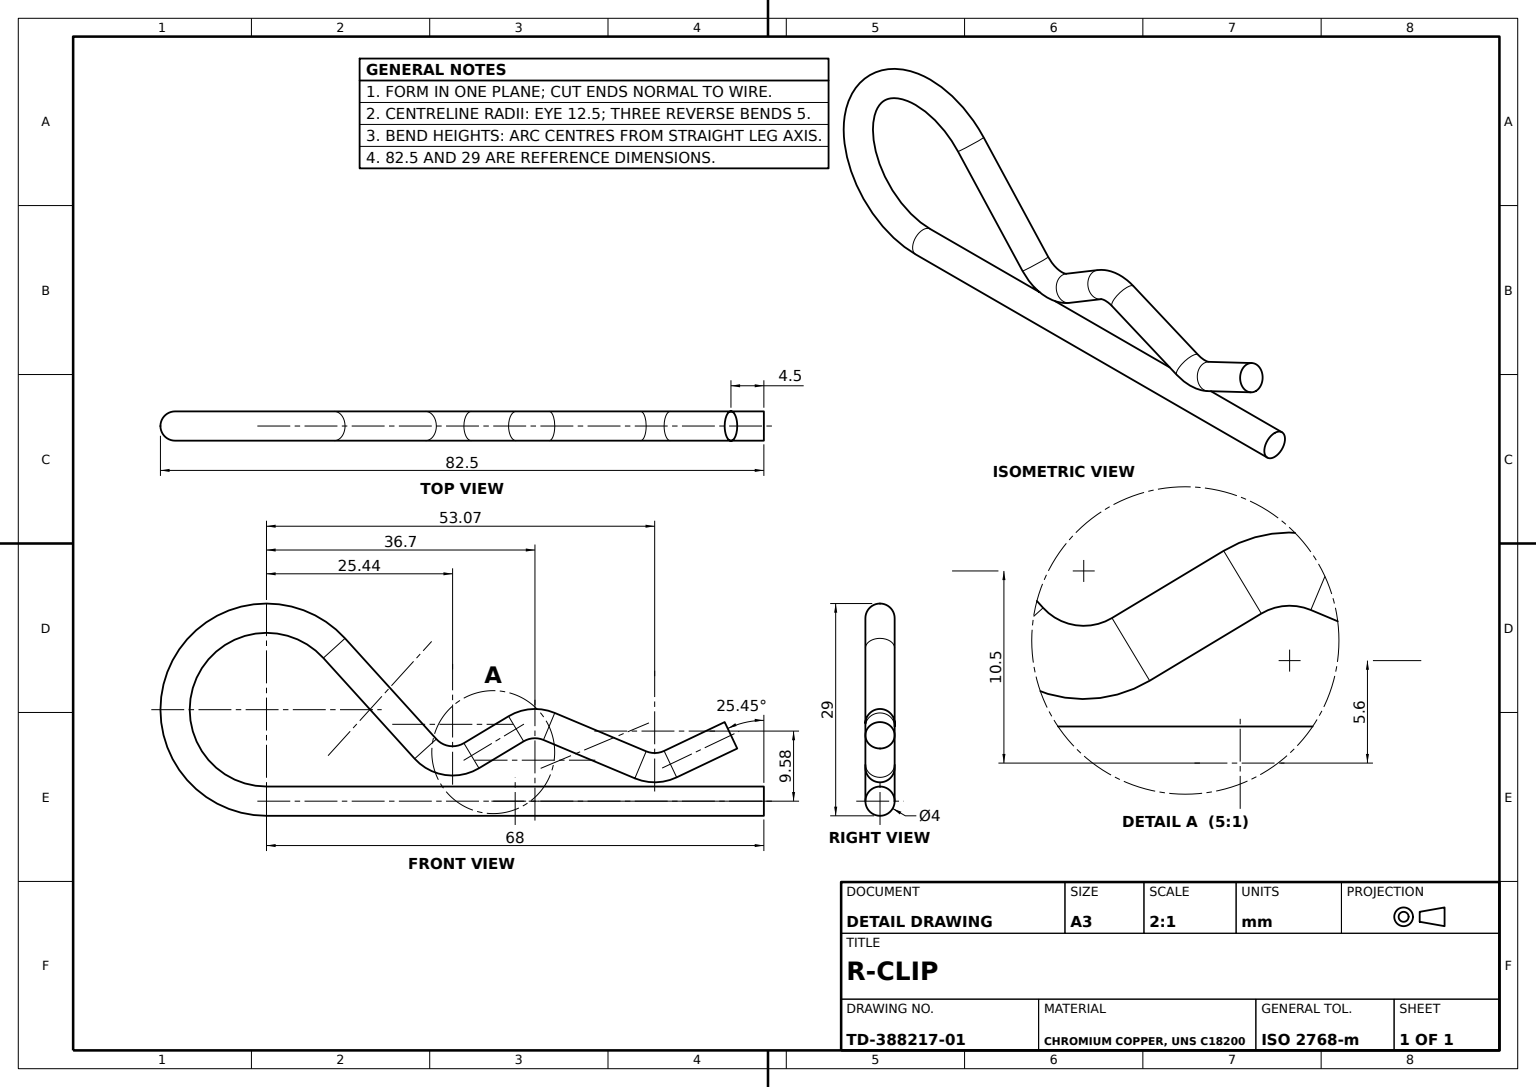
from build123d import *

# Parameters (mm, degrees)
WIRE_SWEEP_4_PROFILE_R = 2


with BuildPart() as part:
    # Wire Sweep Ø4: sweep along a path in Clip Wire Path
    with BuildLine(Plane.XY) as wire_sweep_4_path:
        Line((0, 0), (-68, 0))
        ThreePointArc((-68, 0), (-80.5, 12.5), (-68, 25))
        ThreePointArc((-68, 25), (-62.93740019, 23.928914347), (-58.742396863, 20.899213306))
        Line((-58.742396863, 20.899213306), (-46.259260276, 7.140314678))
        ThreePointArc((-46.259260276, 7.140314678), (-43.2855546, 5.553479039), (-39.980410457, 6.214535003))
        Line((-39.980410457, 6.214535003), (-33.8729527, 9.885464997))
        ThreePointArc((-33.8729527, 9.885464997), (-31.656450173, 10.587073207), (-29.362263704, 10.210448754))
        Line((-29.362263704, 10.210448754), (-16.862956001, 4.964827953))
        ThreePointArc((-16.862956001, 4.964827953), (-14.811169509, 4.576643597), (-12.779773841, 5.060323807))
        Line((-12.779773841, 5.060323807), (-4.5, 9))
    # Wire Sweep Ø4 profile (on start of the path) → Wire Sweep Ø4 (sweep)
    with BuildSketch(Plane(origin=(0, 0, 0), x_dir=(0, -1, 0), z_dir=(-1, 0, 0))):
        Circle(WIRE_SWEEP_4_PROFILE_R)
    sweep(path=wire_sweep_4_path.line)


solid = part.part
